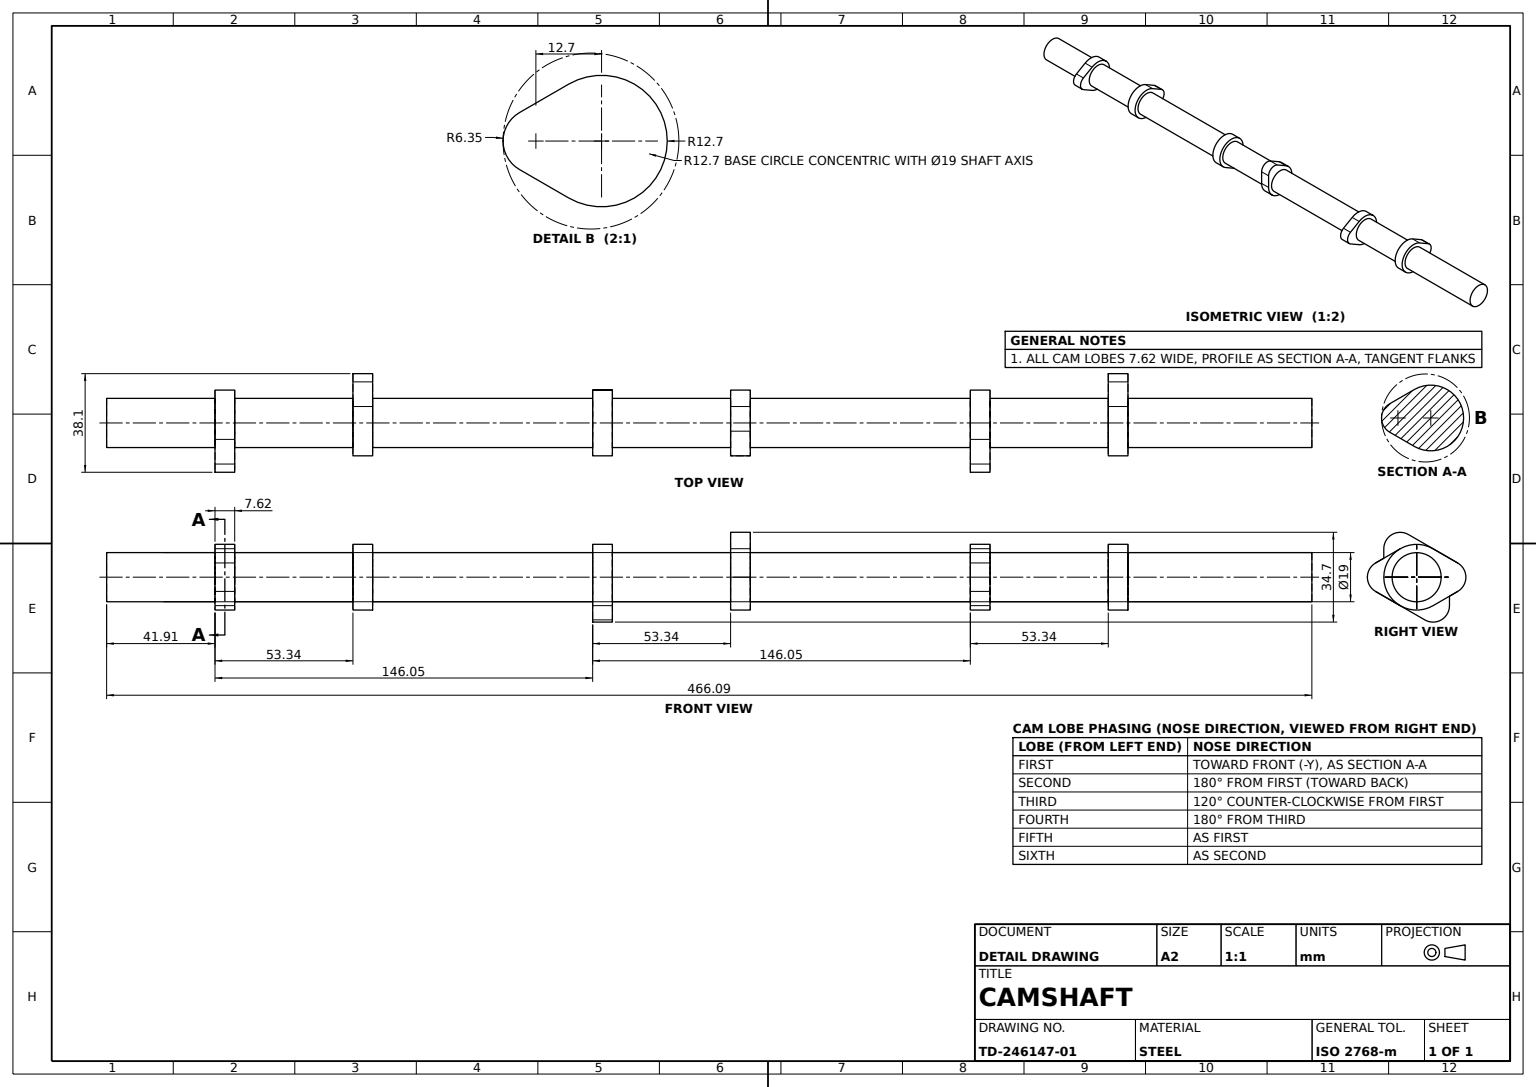
from build123d import *

# Parameters (mm, degrees)
CAM_LOBE_DEPTH                 = 7.62
CAM_LOBE_PAIR_PATTERN_2X_COUNT = 2
CAM_LOBE_PAIR_PATTERN_2X_PITCH = 53.34
ROTATE_LOBE_180DEG_ANGLE       = 180
LOBE_SET_PATTERN_3X_COUNT      = 3
LOBE_SET_PATTERN_3X_PITCH      = 146.05
ROTATE_LOBE_SET_120DEG_ANGLE   = 120
CAMSHAFT_START                 = 49.53
SHAFT_PROFILE_SKETCH_R         = 9.5
CAMSHAFT_SHAFT_DEPTH           = 466.09


with BuildPart() as part:
    # Cam Lobe Profile Sketch → Cam Lobe (new body)
    with BuildSketch(Plane(origin=(0, 0, 0), x_dir=(1, 0, 0), z_dir=(0, 1, 0))):
        with BuildLine():
            Line((-5.499261314, 15.875), (-10.998522628, 6.35))
            ThreePointArc((-10.998522628, 6.35), (0, -12.7), (10.998522628, 6.35))
            Line((10.998522628, 6.35), (5.499261314, 15.875))
            ThreePointArc((5.499261314, 15.875), (0, 19.05), (-5.499261314, 15.875))
        make_face()
    extrude(amount=CAM_LOBE_DEPTH)


with BuildPart() as cam_lobe_pair_pattern_2x_1:
    # Cam Lobe Pair Pattern 2x: pattern copy
    add(part.part.moved(Location(Vector(0, -1, 0) * (1 * CAM_LOBE_PAIR_PATTERN_2X_PITCH))))


with BuildPart() as cam_lobe_pair_pattern_2x_1_1:
    # Rotate Lobe 180deg: moved
    add(cam_lobe_pair_pattern_2x_1.part.rotate(Axis((0, 0, 0), (0, 1, 0)), ROTATE_LOBE_180DEG_ANGLE))


with BuildPart() as lobe_set_pattern_3x_1:
    # Lobe Set Pattern 3x: pattern copy
    add(part.part.moved(Location(Vector(0, -1, 0) * (1 * LOBE_SET_PATTERN_3X_PITCH))))


with BuildPart() as lobe_set_pattern_3x_2:
    # Lobe Set Pattern 3x: pattern copy
    add(part.part.moved(Location(Vector(0, -1, 0) * (2 * LOBE_SET_PATTERN_3X_PITCH))))


with BuildPart() as lobe_set_pattern_3x_3:
    # Lobe Set Pattern 3x: pattern copy
    add(cam_lobe_pair_pattern_2x_1_1.part.moved(Location(Vector(0, -1, 0) * (1 * LOBE_SET_PATTERN_3X_PITCH))))


with BuildPart() as lobe_set_pattern_3x_4:
    # Lobe Set Pattern 3x: pattern copy
    add(cam_lobe_pair_pattern_2x_1_1.part.moved(Location(Vector(0, -1, 0) * (2 * LOBE_SET_PATTERN_3X_PITCH))))


with BuildPart() as lobe_set_pattern_3x_1_1:
    # Rotate Lobe Set 120deg: moved
    add(lobe_set_pattern_3x_1.part.rotate(Axis((0, 0, 0), (0, -1, 0)), ROTATE_LOBE_SET_120DEG_ANGLE))


with BuildPart() as lobe_set_pattern_3x_3_1:
    # Rotate Lobe Set 120deg: moved
    add(lobe_set_pattern_3x_3.part.rotate(Axis((0, 0, 0), (0, -1, 0)), ROTATE_LOBE_SET_120DEG_ANGLE))


with BuildPart() as part_1:
    add(part.part)

    add(cam_lobe_pair_pattern_2x_1_1.part)  # Camshaft Shaft merges Cam Lobe Pair Pattern 2x_1

    add(lobe_set_pattern_3x_1_1.part)  # Camshaft Shaft merges Lobe Set Pattern 3x_1

    add(lobe_set_pattern_3x_2.part)  # Camshaft Shaft merges Lobe Set Pattern 3x_2

    add(lobe_set_pattern_3x_3_1.part)  # Camshaft Shaft merges Lobe Set Pattern 3x_3

    add(lobe_set_pattern_3x_4.part)  # Camshaft Shaft merges Lobe Set Pattern 3x_4
    # Shaft Profile Sketch → Camshaft Shaft (add)
    with BuildSketch(Plane(origin=(0, 0, 0), x_dir=(1, 0, 0), z_dir=(0, 1, 0)).offset(CAMSHAFT_START)):
        with Locations(Location((0, 0, 0), (0, 0, 270))):
            Circle(SHAFT_PROFILE_SKETCH_R)
    extrude(amount=-CAMSHAFT_SHAFT_DEPTH)


solid = part_1.part
